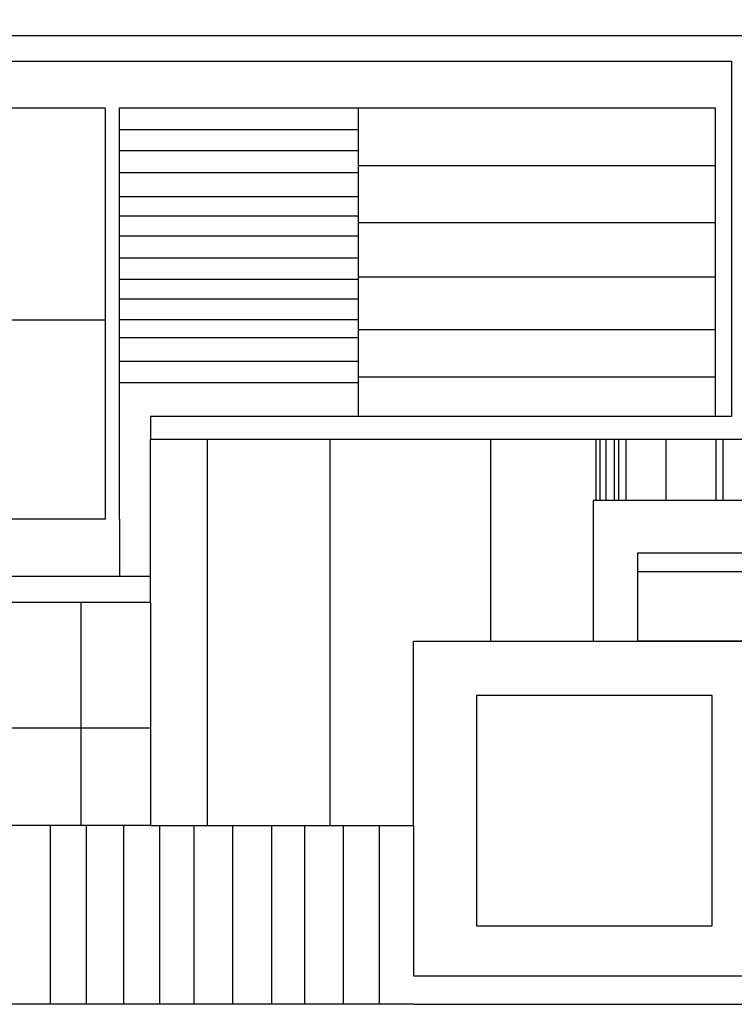
# Model space of a CAD drawing. Units: inches. Extents: x -117 to 121, y -77 to 40.
# Tile 31 of 45: x 34.28 to 47.47, y -7.88 to 10.29. Entities that reach past the tile are written whole.
import ezdxf

# ---------------------------------------------------------------- set-up
doc = ezdxf.new("R2010")
doc.units = ezdxf.units.IN
doc.header["$MEASUREMENT"] = 0
doc.layers.add('A-ANNO-DIMS', color=2, linetype='Continuous', lineweight=18)
doc.layers.add('A-ELEV', color=7, linetype='Continuous', lineweight=25)
doc.styles.get("Standard").update_dxf_attribs({"font": 'arial.ttf'})
doc.dimstyles.get("Standard").update_dxf_attribs({"dimtxt": 0.18, "dimasz": 0.18, "dimexe": 0.18, "dimexo": 0.0625, "dimgap": 0.09, "dimtad": 0, "dimtih": 1, "dimtoh": 1, "dimdec": 4, "dimzin": 0, "dimdsep": 46, "dimtxsty": 'Standard', "dimcen": 0.09, "dimadec": 0, "dimazin": 0, "dimtfac": 1, "dimtdec": 4, "dimtofl": 0, "dimtmove": 0, "dimatfit": 3, "dimfxl": 1, "dimtolj": 1, "dimtzin": 0, "dimarcsym": 0})

# ---------------------------------------------------------------- blocks, each defined once
blk = doc.blocks.new('*D53')
at = {"layer": 'A-ANNO-DIMS', "color": 0, "lineweight": -2, "transparency": 16777216}
for p, q in [((27.974, 10.841), (27.974, -77.193)), ((51.69, 10.9), (51.69, -77.193)), ((28.154, -77.013), (39.367, -77.013)), ((51.51, -77.013), (40.297, -77.013))]:
    blk.add_line(p, q, dxfattribs=at)
at = {"layer": 'A-ANNO-DIMS', "color": 0, "transparency": 16777216}
for points in [[(28.154, -76.983), (28.154, -77.043), (27.974, -77.013)], [(51.51, -76.983), (51.51, -77.043), (51.69, -77.013)]]:
    blk.add_solid(points, dxfattribs=at)
at = {"layer": 'Defpoints', "color": 0, "transparency": 16777216}
for p in [(51.69, 10.962), (27.974, 10.903), (51.69, -77.013)]:
    blk.add_point(p, dxfattribs=at)
at = {"layer": 'A-ANNO-DIMS', "color": 0, "transparency": 16777216, "insert": (39.832, -77.013), "char_height": 0.18, "attachment_point": 5}
blk.add_mtext('\\A1;23.716', dxfattribs=at)

msp = doc.modelspace()

# ---------------------------------------------------------------- linework, layer by layer
at = {"layer": 'A-ELEV'}
for p, q in [((27.8529, 9.9998), (57.6104, 9.9998)), ((28.3319, 9.5278), (47.4236, 9.5278)), ((47.4236, 9.5278), (47.4236, 2.969)), ((29.2247, 8.6669), (35.5042, 8.6669)), ((35.5042, 8.6669), (35.8598, 8.6669)), ((35.8598, 8.6669), (35.8598, 1.0726)), ((36.1266, 1.0726), (36.1266, 8.6669)), ((36.1266, 8.6669), (47.1207, 8.6669)), ((40.532, 8.6669), (40.532, 2.969)), ((47.1207, 8.6669), (47.1207, 2.969)), ((36.1266, 8.2634), (40.532, 8.2634)), ((36.1266, 7.8792), (40.532, 7.8792)), ((36.1266, 7.4709), (40.532, 7.4709)), ((40.532, 7.6039), (47.1207, 7.6039)), ((36.1266, 7.0307), (40.532, 7.0307)), ((36.1266, 6.6687), (40.532, 6.6687)), ((40.532, 6.5457), (47.1207, 6.5457)), ((36.1266, 6.3005), (40.532, 6.3005)), ((36.1266, 5.8972), (40.532, 5.8972)), ((36.1266, 5.505), (40.532, 5.505)), ((40.532, 5.5486), (47.1207, 5.5486)), ((36.1266, 5.1368), (40.532, 5.1368)), ((28.8053, 4.7497), (35.8598, 4.7497)), ((36.1266, 4.7606), (40.532, 4.7606)), ((40.532, 4.5718), (47.1207, 4.5718)), ((36.1266, 4.4244), (40.532, 4.4244)), ((36.1266, 3.9893), (40.532, 3.9893)), ((40.532, 3.6967), (47.1207, 3.6967)), ((36.1266, 3.5971), (40.532, 3.5971)), ((47.4236, 2.969), (36.6962, 2.969)), ((36.6962, 2.969), (36.6962, 2.5428)), ((47.9835, 2.5428), (36.6962, 2.5428)), ((36.6962, -0.458), (36.6962, 2.5428)), ((37.7468, -4.5859), (37.7468, 2.5428)), ((40.0116, -4.5859), (40.0116, 2.5428)), ((42.9798, -1.1791), (42.9798, 2.5428)), ((44.9209, 1.4169), (44.9209, 2.5428)), ((45, 1.4169), (45, 2.5428)), ((45.1055, 1.4169), (45.1055, 2.5428)), ((45.2637, 1.4169), (45.2637, 2.5428)), ((45.3429, 1.4169), (45.3429, 2.5428)), ((45.4747, 1.4169), (45.4747, 2.5428)), ((46.2132, 1.4169), (46.2132, 2.5428)), ((47.1363, 1.4169), (47.1363, 2.5428)), ((47.2682, 1.4169), (47.2682, 2.5428)), ((57.6104, 1.4169), (44.867, 1.4169)), ((44.867, 1.4169), (44.867, -1.1791)), ((35.8598, 1.0726), (28.8053, 1.0726)), ((36.1266, 1.0726), (36.1266, 0.0223)), ((45.6904, -1.1791), (45.6904, 0.4475)), ((45.6904, 0.4475), (57.6104, 0.4475)), ((28.3319, 0.0223), (36.6962, 0.0223)), ((45.6904, 0.1069), (57.6104, 0.1069)), ((27.8529, -0.458), (36.6962, -0.458)), ((35.4128, -0.458), (35.4128, -4.5859)), ((36.6962, -0.458), (36.6962, -4.5859)), ((41.553, -4.5859), (41.553, -1.1791)), ((41.553, -1.1791), (48.069, -1.1791)), ((57.6104, -1.1791), (45.6904, -1.1791)), ((42.7148, -2.1844), (42.7148, -6.4341)), ((47.062, -2.1844), (42.7148, -2.1844)), ((47.062, -6.4341), (47.062, -2.1844)), ((24.2772, -2.7834), (36.6962, -2.7834)), ((36.6962, -4.5859), (24.2772, -4.5859)), ((34.8472, -4.5859), (34.8472, -7.8846)), ((35.5094, -4.5859), (35.5094, -7.8846)), ((36.1993, -4.5859), (36.1993, -7.8846)), ((36.6962, -4.5859), (37.7468, -4.5859)), ((36.8616, -4.5859), (36.8616, -7.8846)), ((37.4962, -4.5859), (37.4962, -7.8846)), ((37.7468, -4.5859), (41.553, -4.5859)), ((38.2137, -4.5859), (38.2137, -7.8846)), ((38.9311, -4.5859), (38.9311, -7.8846)), ((39.5382, -4.5859), (39.5382, -7.8846)), ((40.2556, -4.5859), (40.2556, -7.8846)), ((40.9179, -4.5859), (40.9179, -7.8846)), ((41.553, -4.5859), (41.553, -6.5943)), ((42.7148, -6.4341), (47.062, -6.4341)), ((41.553, -6.5943), (41.553, -7.3579)), ((41.553, -7.3579), (48.069, -7.3579)), ((41.553, -7.8846), (24.2772, -7.8846)), ((41.553, -7.8846), (57.6104, -7.8846))]:
    msp.add_line(p, q, dxfattribs=at)

# ---------------------------------------------------------------- dimensions: what is measured, and where the dimension line sits
at = {"layer": 'A-ANNO-DIMS'}
dim = msp.add_linear_dim(base=(51.6901, -77.0135), p1=(27.9744, 10.9032), p2=(51.6901, 10.9623), dimstyle='Standard', override={"dimdec": 3, "dimlfac": 1, "dimrnd": 0, "dimzin": 0, "dimdsep": 46, "dimlunit": 2}, dxfattribs=at)
dim.commit()
dim.dimension.update_dxf_attribs({"geometry": '*D53', "text_midpoint": (39.8322, -77.0135)})

doc.saveas('drawing.dxf')
